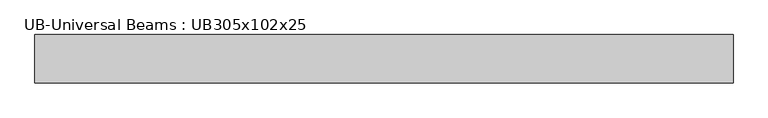
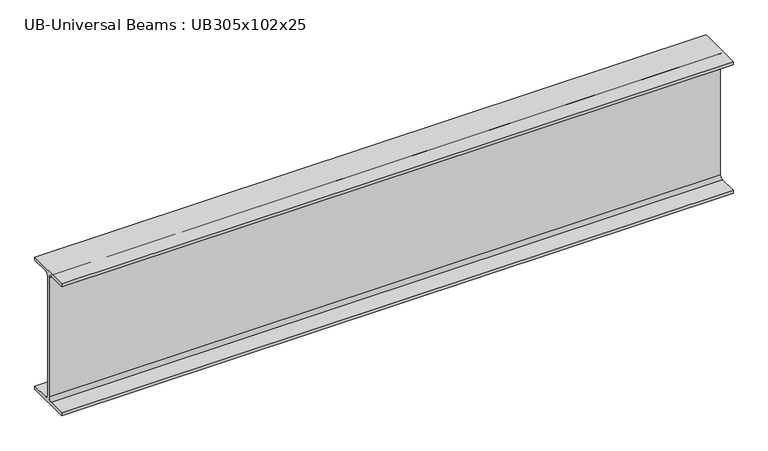
"""IFC4 building model written with IfcOpenShell, lengths in millimetres: beam geometry, UB-Universal Beams : UB305x102x25."""

from ifc_helpers import new_model, si_unit, point, frame, frame_2d, origin, place, context, project, spatial, polyline, circle_curve, trimmed, segment, composite_curve, outline, extrude, source, transform, mapped, element, save


def ub_universal_beams_ub305x102x25_1ef2d586(model_context):
    return source(origin(), model_context, "Body", "SweptSolid", [
        extrude(outline(composite_curve([segment(polyline([(50.8, -145.55), (50.8, -152.55), (-50.8, -152.55), (-50.8, -145.55), (-10.5, -145.55)]), True, "CONTINUOUS"), segment(trimmed(circle_curve(frame_2d((-10.5, -137.95)), 7.6), [point((-10.5, -145.55))], [point((-2.9, -137.95))], True, "CARTESIAN"), True, "CONTINUOUS"), segment(polyline([(-2.9, -137.95), (-2.9, 137.95)]), True, "CONTINUOUS"), segment(trimmed(circle_curve(frame_2d((-10.5, 137.95)), 7.6), [point((-2.9, 137.95))], [point((-10.5, 145.55))], True, "CARTESIAN"), True, "CONTINUOUS"), segment(polyline([(-10.5, 145.55), (-50.8, 145.55), (-50.8, 152.55), (50.8, 152.55), (50.8, 145.55), (10.5, 145.55)]), True, "CONTINUOUS"), segment(trimmed(circle_curve(frame_2d((10.5, 137.95)), 7.6), [point((10.5, 145.55))], [point((2.9, 137.95))], True, "CARTESIAN"), True, "CONTINUOUS"), segment(polyline([(2.9, 137.95), (2.9, -137.95)]), True, "CONTINUOUS"), segment(trimmed(circle_curve(frame_2d((10.5, -137.95)), 7.6), [point((2.9, -137.95))], [point((10.5, -145.55))], True, "CARTESIAN"), True, "CONTINUOUS"), segment(polyline([(10.5, -145.55), (50.8, -145.55)]), True, "CONTINUOUS")], self_intersect=False)), frame((-734.7, 0.0, 0.0), z_axis=(1.0, 0.0, 0.0), x_axis=(0.0, 1.0, 0.0)), (0.0, 0.0, 1.0), 1469.4),
    ])


if __name__ == "__main__":
    model = new_model("IFC4")
    model_context = context("Model", 3, world=origin())
    ifc_project = project(units=[si_unit("LENGTHUNIT", "METRE", prefix="MILLI")], contexts=[model_context])
    site = spatial("IfcSite", under=ifc_project)
    building = spatial("IfcBuilding", under=site)
    placement = place(None, origin())
    ub_universal_beams_ub305x102x25_shape = ub_universal_beams_ub305x102x25_1ef2d586(model_context)
    element("IfcBeam", 1, ObjectType="UB-Universal Beams : UB305x102x25", at=placement, inside=building, context=model_context, shape_type="MappedRepresentation", body=[
        mapped(ub_universal_beams_ub305x102x25_shape, transform((0.0, 0.0, 0.0), x_axis=(1.0, 0.0, 0.0), y_axis=(0.0, 1.0, 0.0), z_axis=(0.0, 0.0, 1.0))),
    ])
    save(model, "model.ifc")

# Revit data of these elements
# Type "UB-Universal Beams : UB305x102x25"
#   Section Name Key = "UB305X102X25"
#   Width = 10.16 cm
#   Web Thickness = 0.58 cm
#   Web Fillet = 0.76 cm
#   Warping Constant = 27300.0 cm⁶
#   Torsional Moment of Inertia = 4.77 cm⁴
#   Section Area = 31.6 cm²
#   Plastic Modulus weak axis = 39.0 cm³
#   Plastic Modulus strong axis = 342.0 cm³
#   Nominal Weight = 24.7999 kgf/m
#   Moment of Inertia weak axis = 123.00 cm⁴
#   Moment of Inertia strong axis = 4455.00 cm⁴
#   Height = 30.51 cm
#   Flange Thickness = 0.7 cm
#   Elastic Modulus weak axis = 24.2 cm³
#   Elastic Modulus strong axis = 292.0 cm³
#   Centroid Vertical = 15.255 cm
#   Centroid Horizontal = 5.08 cm
#   Bolt Spacing = 5.4 cm
#   Length [instance default] = 1.5 m
#   Structural Material [instance default] = Metal - Steel 43-275
#   Type Comments = ""
#   Assembly Code = ""
# Element 1 (IfcBeam, "UB-Universal Beams : UB305x102x25")
#   Materials on its faces: "Metal - Steel 43-275"
# Materials
#   "Metal - Steel 43-275": class "Metal", colour RGB 247 247 247, transparency 0, Cost = 0
